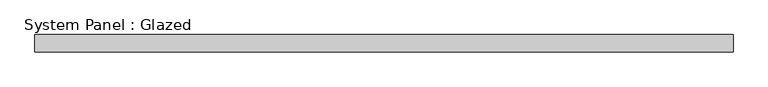
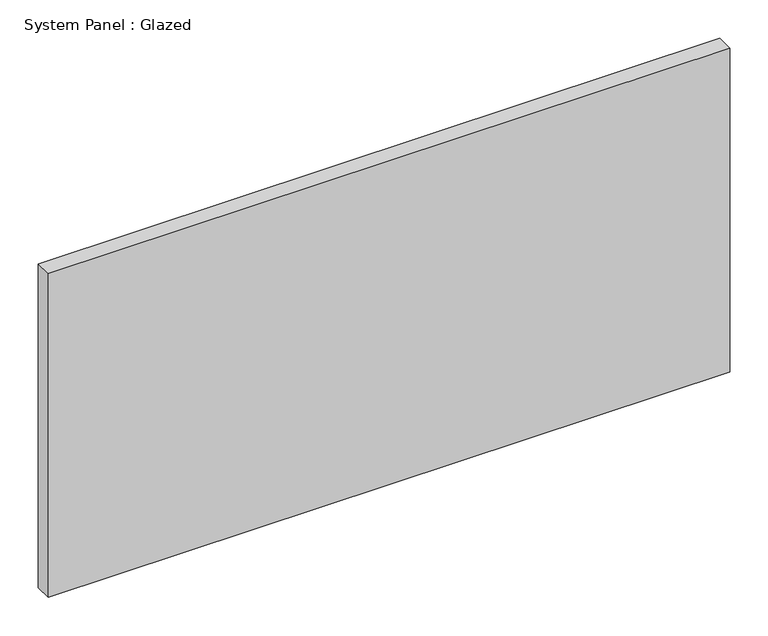
"""IFC4 building model written with IfcOpenShell, lengths in millimetres: plate geometry, System Panel : Glazed."""

from ifc_helpers import new_model, si_unit, origin, origin_with_axes, place, context, project, spatial, polyline, outline, extrude, source, transform, mapped, element, save


def system_panel_glazed_6663e6a9(model_context):
    return source(origin(), model_context, "Body", "SweptSolid", [
        extrude(outline(polyline([(511.175, 19.05), (-511.175, 19.05), (-511.175, 44.45), (511.175, 44.45), (511.175, 19.05)])), origin_with_axes(), (0.0, 0.0, 1.0), 514.35),
    ])


if __name__ == "__main__":
    model = new_model("IFC4")
    model_context = context("Model", 3, world=origin())
    ifc_project = project(units=[si_unit("LENGTHUNIT", "METRE", prefix="MILLI")], contexts=[model_context])
    site = spatial("IfcSite", under=ifc_project)
    building = spatial("IfcBuilding", under=site)
    placement = place(None, origin())
    system_panel_glazed_shape = system_panel_glazed_6663e6a9(model_context)
    element("IfcPlate", 1, ObjectType="System Panel : Glazed", at=placement, inside=building, context=model_context, shape_type="MappedRepresentation", body=[
        mapped(system_panel_glazed_shape, transform((0.0, 0.0, 0.0), x_axis=(1.0, 0.0, 0.0), y_axis=(0.0, 1.0, 0.0), z_axis=(0.0, 0.0, 1.0))),
    ])
    save(model, "model.ifc")

# Revit data of these elements
# Type "System Panel : Glazed"
#   Construction Type Id = "GSP4R"
#   Analytic Construction = "1/8 in Pilkington single glazing"
#   Visual Light Transmittance = 0.9
#   Solar Heat Gain Coefficient = 0.86
#   Heat Transfer Coefficient (U) = 1.18115 BTU/(h·ft²·°F)
# Element 1 (IfcPlate, "System Panel : Glazed")
#   Materials on its faces: "Glass"
# Materials
#   "Glass": class "Glass", colour RGB 0 128 192, transparency 0.75, Description = "Soda Lime Glass", Cost = 0
